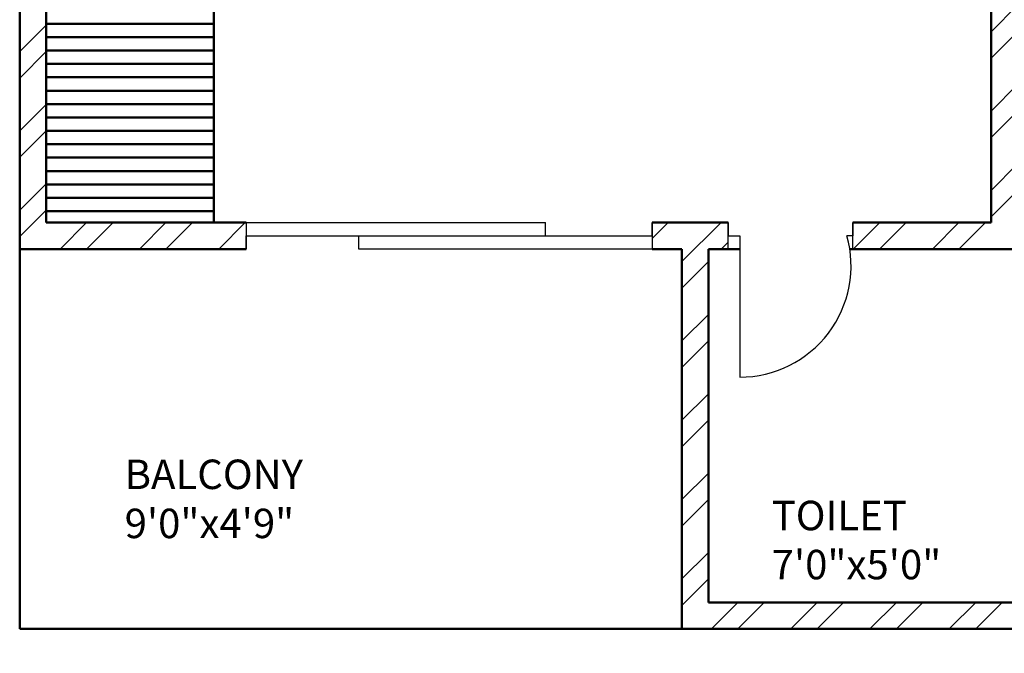
# Model space of a CAD drawing. Units: inches. Extents: x 963 to 2075, y 289 to 2657.
# Tile 1 of 98: x 1091 to 1259, y 1474 to 1582. Entities that reach past the tile are written whole.
import ezdxf

# ---------------------------------------------------------------- set-up
doc = ezdxf.new("R2010")
doc.units = ezdxf.units.IN
for name, color, linetype, lineweight in [('A-AREA-IDEN', 7, 'Continuous', 18), ('A-DOOR', 4, 'Continuous', 25), ('A-GLAZ', 3, 'Continuous', 25), ('A-WALL', 7, 'Continuous', 50), ('A-WALL-PATT', 8, 'Continuous', 13)]:
    doc.layers.add(name, color=color, linetype=linetype, lineweight=lineweight)
doc.styles.get("Standard").update_dxf_attribs({"font": 'arial.ttf'})

msp = doc.modelspace()

# ---------------------------------------------------------------- hatches: boundary and pattern name
at = {"layer": 'A-WALL-PATT'}
h = msp.add_hatch(dxfattribs=at)
h.set_pattern_fill('ANSI32', color=256)
h.paths.add_polyline_path([(1296.92, 2558.32), (1203.92, 2558.32), (1203.92, 2493.82), (1191.53, 2493.82), (1191.53, 2489.32), (1211.06, 2489.32), (1211.06, 2492.02), (1211.06, 2493.82), (1208.42, 2493.82), (1208.42, 2553.82), (1292.42, 2553.82), (1292.42, 2538.86), (1296.92, 2538.86)])
h.paths.add_polyline_path([(1442.42, 2558.32), (1349.42, 2558.32), (1349.42, 2538.94), (1353.92, 2538.94), (1353.92, 2553.82), (1437.92, 2553.82), (1437.92, 2493.82), (1434.54, 2493.82), (1434.54, 2489.32), (1448.31, 2489.32), (1448.31, 2491.57), (1448.31, 2493.82), (1442.42, 2493.82)])
h.paths.add_polyline_path([(1415.55, 2491.57), (1415.55, 2493.82), (1340.94, 2493.82), (1340.94, 2489.32), (1371.92, 2489.32), (1371.92, 2378.32), (1367.6, 2378.32), (1367.6, 2373.82), (1371.92, 2373.82), (1371.92, 2355.19), (1376.42, 2355.19), (1376.42, 2489.32), (1415.55, 2489.32)])
h.paths.add_polyline_path([(1304.94, 2491.57), (1304.94, 2493.82), (1296.92, 2493.82), (1296.92, 2514.86), (1292.42, 2514.86), (1292.42, 2493.82), (1232.81, 2493.82), (1232.81, 2489.32), (1256.42, 2489.32), (1256.42, 2327.32), (1253.71, 2327.32), (1253.71, 2322.82), (1328.42, 2322.82), (1328.42, 2331.15), (1323.92, 2331.15), (1323.92, 2327.32), (1260.92, 2327.32), (1260.92, 2373.82), (1323.92, 2373.82), (1323.92, 2357.81), (1328.42, 2357.81), (1328.42, 2373.82), (1346.01, 2373.82), (1346.01, 2376.07), (1346.01, 2378.32), (1260.92, 2378.32), (1260.92, 2489.32), (1304.94, 2489.32)])
h.paths.add_polyline_path([(1226.65, 2327.32), (1124.42, 2327.32), (1124.42, 2347.45), (1119.92, 2347.45), (1119.92, 2322.82), (1163.42, 2322.82), (1163.42, 2305.43), (1165.67, 2305.43), (1167.92, 2305.43), (1167.92, 2322.82), (1226.65, 2322.82), (1226.65, 2325.07)])
h.paths.add_polyline_path([(1095.92, 2489.32), (1124.42, 2489.32), (1131.53, 2489.32), (1131.53, 2491.57), (1131.53, 2493.82), (1119.92, 2493.82), (1091.42, 2493.82), (1091.42, 2417.32), (1095.92, 2417.32), (1119.92, 2417.32), (1119.92, 2407.45), (1124.42, 2407.45), (1124.42, 2421.82), (1095.92, 2421.82)])
h.paths.add_polyline_path([(1512.92, 2558.32), (1508.42, 2558.32), (1508.42, 2493.82), (1503.4, 2493.82), (1503.4, 2489.32), (1508.42, 2489.32), (1508.42, 2327.32), (1376.42, 2327.32), (1376.42, 2330.27), (1371.92, 2330.27), (1371.92, 2298.74), (1376.42, 2298.74), (1376.42, 2322.82), (1508.42, 2322.82), (1508.42, 2165.32), (1504.26, 2165.32), (1504.26, 2160.82), (1508.42, 2160.82), (1508.42, 2108.32), (1512.92, 2108.32), (1512.92, 2160.82), (1516.18, 2160.82), (1516.18, 2163.07), (1516.18, 2165.32), (1512.92, 2165.32), (1512.92, 2322.82), (1644.92, 2322.82), (1644.92, 2298.74), (1649.42, 2298.74), (1649.42, 2322.82), (1649.42, 2330.94), (1647.17, 2330.94), (1644.92, 2330.94), (1644.92, 2327.32), (1512.92, 2327.32), (1512.92, 2489.32), (1516.76, 2489.32), (1516.76, 2491.57), (1516.76, 2493.82), (1512.92, 2493.82)])
h.paths.add_polyline_path([(1671.92, 2558.32), (1578.92, 2558.32), (1578.92, 2493.82), (1573.53, 2493.82), (1573.53, 2489.32), (1586.54, 2489.32), (1586.54, 2491.57), (1586.54, 2493.82), (1583.42, 2493.82), (1583.42, 2553.82), (1667.42, 2553.82), (1667.42, 2541.11), (1671.92, 2541.11)])
h.paths.add_polyline_path([(1681.26, 2493.82), (1671.92, 2493.82), (1671.92, 2517.11), (1667.42, 2517.11), (1667.42, 2493.82), (1610.22, 2493.82), (1610.22, 2489.32), (1644.92, 2489.32), (1644.92, 2357.87), (1649.42, 2357.87), (1649.42, 2373.82), (1652.2, 2373.82), (1652.2, 2375.83), (1652.2, 2378.32), (1649.42, 2378.32), (1649.42, 2489.32), (1681.26, 2489.32), (1681.26, 2491.57)])
h.paths.add_polyline_path([(1821.92, 2558.32), (1728.92, 2558.32), (1728.92, 2541), (1733.42, 2541), (1733.42, 2553.82), (1817.42, 2553.82), (1817.42, 2493.82), (1813.51, 2493.82), (1813.51, 2489.32), (1830.08, 2489.32), (1830.08, 2491.57), (1830.08, 2493.82), (1821.92, 2493.82)])
h.paths.add_polyline_path([(1794.24, 2493.82), (1717.26, 2493.82), (1717.26, 2489.32), (1760.42, 2489.32), (1760.42, 2378.32), (1674.4, 2378.32), (1674.4, 2373.82), (1692.92, 2373.82), (1692.92, 2356.95), (1697.42, 2356.95), (1697.42, 2373.82), (1760.42, 2373.82), (1760.42, 2327.32), (1697.42, 2327.32), (1697.42, 2333.34), (1692.92, 2333.34), (1692.92, 2322.82), (1768.04, 2322.82), (1768.04, 2325.07), (1768.04, 2327.32), (1764.92, 2327.32), (1764.92, 2489.32), (1794.24, 2489.32)])
h.paths.add_polyline_path([(1733.42, 2517), (1728.92, 2517), (1728.92, 2493.82), (1733.42, 2493.82)], flags=17)
h.paths.add_polyline_path([(1929.92, 2493.82), (1890.08, 2493.82), (1890.08, 2489.32), (1896.92, 2489.32), (1925.42, 2489.32), (1925.42, 2421.82), (1896.92, 2421.82), (1896.92, 2408.32), (1901.42, 2408.32), (1901.42, 2417.32), (1925.42, 2417.32), (1929.92, 2417.32)])
h.paths.add_polyline_path([(1901.42, 2348.32), (1896.92, 2348.32), (1896.92, 2327.32), (1800.42, 2327.32), (1800.42, 2322.82), (1853.42, 2322.82), (1853.42, 2309.45), (1857.92, 2309.45), (1857.92, 2322.82), (1901.42, 2322.82)])
h.paths.add_polyline_path([(1857.92, 2249.45), (1853.42, 2249.45), (1853.42, 2214.82), (1686.31, 2214.82), (1686.31, 2210.32), (1853.42, 2210.32), (1853.42, 2202.13), (1857.92, 2202.13), (1857.92, 2210.32)])
h.paths.add_polyline_path([(1857.92, 2142.13), (1853.42, 2142.13), (1853.42, 2115.42), (1841.42, 2115.42), (1841.42, 2088.53), (1841.42, 2046.95), (1845.92, 2046.95), (1845.92, 2110.92), (1905.92, 2110.92), (1905.92, 2092.52), (1910.42, 2092.52), (1910.42, 2115.42), (1857.92, 2115.42)])
h.paths.add_polyline_path([(1532.44, 1482.34), (1573.46, 1482.34), (1573.46, 1501), (1532.44, 1501)], flags=9)
h.paths.add_polyline_path([(1438.66, 1486.3), (1479.68, 1486.3), (1479.68, 1504.96), (1438.66, 1504.96)], flags=9)
h.paths.add_polyline_path([(1411.22, 1365.31), (1659.14, 1365.31), (1659.14, 1402.4), (1411.22, 1402.4)], flags=9)
h.paths.add_polyline_path([(1185.67, 2296.3), (1248.16, 2296.3), (1248.16, 2314.95), (1185.67, 2314.95)], flags=9)
h.paths.add_polyline_path([(1177.31, 2187.35), (1216.15, 2187.35), (1216.15, 2206.01), (1177.31, 2206.01)], flags=9)
h.paths.add_polyline_path([(1295.1, 1602.08), (1328.26, 1602.08), (1328.26, 1620.74), (1295.1, 1620.74)], flags=9)
h.paths.add_polyline_path([(1525.13, 2005.99), (1558.39, 2005.99), (1558.39, 2024.65), (1525.13, 2024.65)], flags=9)
h.paths.add_polyline_path([(1459.61, 1977.13), (1472.19, 1977.13), (1472.19, 1987.43), (1459.61, 1987.43)], flags=9)
h.paths.add_polyline_path([(1467.81, 2053.68), (1480.02, 2053.68), (1480.02, 2063.98), (1467.81, 2063.98)], flags=9)
h.paths.add_polyline_path([(1555.18, 2119.02), (1584.56, 2119.02), (1584.56, 2137.68), (1555.18, 2137.68)], flags=25)
h.paths.add_polyline_path([(1405.39, 2115.29), (1444.48, 2115.29), (1444.48, 2133.95), (1405.39, 2133.95)], flags=25)
h.paths.add_polyline_path([(1698.48, 2004.26), (1727.69, 2004.26), (1727.69, 2022.92), (1698.48, 2022.92)], flags=9)
h.paths.add_polyline_path([(1612.16, 1972.86), (1629.02, 1972.86), (1629.02, 1983.16), (1612.16, 1983.16)], flags=9)
h.paths.add_polyline_path([(1608.29, 2060.04), (1625.15, 2060.04), (1625.15, 2070.34), (1608.29, 2070.34)], flags=9)
h.paths.add_polyline_path([(1527.95, 1684.4), (1566.79, 1684.4), (1566.79, 1703.06), (1527.95, 1703.06)], flags=9)
h.paths.add_polyline_path([(1422.79, 1683.59), (1461.63, 1683.59), (1461.63, 1702.25), (1422.79, 1702.25)], flags=9)
h.paths.add_polyline_path([(1531.26, 1732.46), (1574.01, 1732.46), (1574.01, 1751.12), (1531.26, 1751.12)], flags=9)
h.paths.add_polyline_path([(1402.87, 1732.85), (1439.8, 1732.85), (1439.8, 1751.5), (1402.87, 1751.5)], flags=9)
h.paths.add_polyline_path([(1243.12, 1923.13), (1281.96, 1923.13), (1281.96, 1941.79), (1243.12, 1941.79)], flags=9)
h.paths.add_polyline_path([(1181.75, 1792.27), (1244.24, 1792.27), (1244.24, 1810.93), (1181.75, 1810.93)], flags=9)
h.paths.add_polyline_path([(1265.82, 1670.3), (1316.07, 1670.3), (1316.07, 1688.96), (1265.82, 1688.96)], flags=9)
h.paths.add_polyline_path([(1140.26, 1676.05), (1179.1, 1676.05), (1179.1, 1694.71), (1140.26, 1694.71)], flags=9)
h.paths.add_polyline_path([(1107.49, 1490.89), (1143.37, 1490.89), (1143.37, 1509.55), (1107.49, 1509.55)], flags=9)
h.paths.add_polyline_path([(1217.58, 1483.9), (1246.74, 1483.9), (1246.74, 1502.56), (1217.58, 1502.56)], flags=9)
h.paths.add_polyline_path([(1389.21, 1486.92), (1418.37, 1486.92), (1418.37, 1505.58), (1389.21, 1505.58)], flags=9)
h.paths.add_polyline_path([(1672.21, 1602.08), (1705.37, 1602.08), (1705.37, 1620.74), (1672.21, 1620.74)], flags=9)
h.paths.add_polyline_path([(1752.08, 1522.64), (1781.24, 1522.64), (1781.24, 1541.3), (1752.08, 1541.3)], flags=9)
h.paths.add_polyline_path([(1848.27, 1491.26), (1884.16, 1491.26), (1884.16, 1509.92), (1848.27, 1509.92)], flags=9)
h.paths.add_polyline_path([(1822.47, 1685.62), (1861.31, 1685.62), (1861.31, 1704.28), (1822.47, 1704.28)], flags=9)
h.paths.add_polyline_path([(1713.19, 1672.23), (1763.44, 1672.23), (1763.44, 1690.89), (1713.19, 1690.89)], flags=9)
h.paths.add_polyline_path([(1736.62, 1790.58), (1799.11, 1790.58), (1799.11, 1809.24), (1736.62, 1809.24)], flags=9)
h.paths.add_polyline_path([(1691.49, 1916.36), (1730.33, 1916.36), (1730.33, 1935.01), (1691.49, 1935.01)], flags=9)
h.paths.add_polyline_path([(1764.87, 1973.92), (1794.31, 1973.92), (1794.31, 1992.58), (1764.87, 1992.58)], flags=9)
h.paths.add_polyline_path([(1767.85, 2034.02), (1797.29, 2034.02), (1797.29, 2052.67), (1767.85, 2052.67)], flags=9)
h.paths.add_polyline_path([(1851.59, 2060.33), (1880.75, 2060.33), (1880.75, 2078.99), (1851.59, 2078.99)], flags=25)
h.paths.add_polyline_path([(1688.49, 2086.87), (1727.33, 2086.87), (1727.33, 2105.53), (1688.49, 2105.53)], flags=9)
h.paths.add_polyline_path([(1537.74, 2293.58), (1580.49, 2293.58), (1580.49, 2312.24), (1537.74, 2312.24)], flags=25)
h.paths.add_polyline_path([(1425.59, 2296.11), (1468.34, 2296.11), (1468.34, 2314.77), (1425.59, 2314.77)], flags=25)
h.paths.add_polyline_path([(1278.52, 2004.18), (1307.72, 2004.18), (1307.72, 2022.84), (1278.52, 2022.84)], flags=9)
h.paths.add_polyline_path([(1193.28, 1973.63), (1222.72, 1973.63), (1222.72, 1992.29), (1193.28, 1992.29)], flags=9)
h.paths.add_polyline_path([(1192.41, 2040.58), (1221.84, 2040.58), (1221.84, 2059.23), (1192.41, 2059.23)], flags=9)
h.paths.add_polyline_path([(1130.6, 1951.39), (1159.76, 1951.39), (1159.76, 1970.05), (1130.6, 1970.05)], flags=9)
h.paths.add_polyline_path([(1132.83, 2052.49), (1161.98, 2052.49), (1161.98, 2071.15), (1132.83, 2071.15)], flags=9)
h.paths.add_polyline_path([(1265.13, 2334.62), (1315.38, 2334.62), (1315.38, 2353.28), (1265.13, 2353.28)], flags=25)
h.paths.add_polyline_path([(1136.74, 2330.79), (1175.58, 2330.79), (1175.58, 2349.44), (1136.74, 2349.44)], flags=9)
h.paths.add_polyline_path([(1287.42, 2417.2), (1320.58, 2417.2), (1320.58, 2435.86), (1287.42, 2435.86)], flags=25)
h.paths.add_polyline_path([(1430.99, 2329.16), (1469.83, 2329.16), (1469.83, 2347.82), (1430.99, 2347.82)], flags=25)
h.paths.add_polyline_path([(1525.42, 2329.21), (1564.26, 2329.21), (1564.26, 2347.87), (1525.42, 2347.87)], flags=25)
h.paths.add_polyline_path([(1684.52, 2382.8), (1717.68, 2382.8), (1717.68, 2401.46), (1684.52, 2401.46)], flags=25)
h.paths.add_polyline_path([(1704.81, 2340.29), (1755.05, 2340.29), (1755.05, 2358.95), (1704.81, 2358.95)], flags=25)
h.paths.add_polyline_path([(1694.11, 2287.76), (1756.6, 2287.76), (1756.6, 2306.41), (1694.11, 2306.41)], flags=9)
h.paths.add_polyline_path([(1815.78, 2329.86), (1854.62, 2329.86), (1854.62, 2348.52), (1815.78, 2348.52)], flags=9)
h.paths.add_polyline_path([(1842.87, 2514.26), (1878.76, 2514.26), (1878.76, 2532.91), (1842.87, 2532.91)], flags=9)
h.paths.add_polyline_path([(1769.51, 2531.45), (1798.67, 2531.45), (1798.67, 2550.1), (1769.51, 2550.1)], flags=25)
h.paths.add_polyline_path([(1594.77, 2518.47), (1623.93, 2518.47), (1623.93, 2537.13), (1594.77, 2537.13)], flags=25)
h.paths.add_polyline_path([(1520.72, 2516.18), (1556.61, 2516.18), (1556.61, 2534.84), (1520.72, 2534.84)], flags=25)
h.paths.add_polyline_path([(1464.46, 2516.69), (1500.34, 2516.69), (1500.34, 2535.35), (1464.46, 2535.35)], flags=25)
h.paths.add_polyline_path([(1365.7, 2528.97), (1394.85, 2528.97), (1394.85, 2547.63), (1365.7, 2547.63)], flags=25)
h.paths.add_polyline_path([(1222.84, 2516.23), (1252, 2516.23), (1252, 2534.89), (1222.84, 2534.89)], flags=25)
h.paths.add_polyline_path([(1104.55, 2509.6), (1140.43, 2509.6), (1140.43, 2528.26), (1104.55, 2528.26)], flags=9)
h = msp.add_hatch(dxfattribs=at)
h.set_pattern_fill('ANSI32', color=256)
h.paths.add_polyline_path([(1335.97, 2212.57), (1335.97, 2214.82), (1167.92, 2214.82), (1167.92, 2245.43), (1163.42, 2245.43), (1163.42, 2210.32), (1163.42, 2194.81), (1167.92, 2194.81), (1167.92, 2210.32), (1335.97, 2210.32)])
h.paths.add_polyline_path([(1532.44, 1482.34), (1573.46, 1482.34), (1573.46, 1501), (1532.44, 1501)], flags=9)
h.paths.add_polyline_path([(1438.66, 1486.3), (1479.68, 1486.3), (1479.68, 1504.96), (1438.66, 1504.96)], flags=9)
h.paths.add_polyline_path([(1411.22, 1365.31), (1659.14, 1365.31), (1659.14, 1402.4), (1411.22, 1402.4)], flags=9)
h.paths.add_polyline_path([(1185.67, 2296.3), (1248.16, 2296.3), (1248.16, 2314.95), (1185.67, 2314.95)], flags=9)
h.paths.add_polyline_path([(1177.31, 2187.35), (1216.15, 2187.35), (1216.15, 2206.01), (1177.31, 2206.01)], flags=9)
h.paths.add_polyline_path([(1295.1, 1602.08), (1328.26, 1602.08), (1328.26, 1620.74), (1295.1, 1620.74)], flags=9)
h.paths.add_polyline_path([(1525.13, 2005.99), (1558.39, 2005.99), (1558.39, 2024.65), (1525.13, 2024.65)], flags=9)
h.paths.add_polyline_path([(1459.61, 1977.13), (1472.19, 1977.13), (1472.19, 1987.43), (1459.61, 1987.43)], flags=9)
h.paths.add_polyline_path([(1467.81, 2053.68), (1480.02, 2053.68), (1480.02, 2063.98), (1467.81, 2063.98)], flags=9)
h.paths.add_polyline_path([(1555.18, 2119.02), (1584.56, 2119.02), (1584.56, 2137.68), (1555.18, 2137.68)], flags=9)
h.paths.add_polyline_path([(1405.39, 2115.29), (1444.48, 2115.29), (1444.48, 2133.95), (1405.39, 2133.95)], flags=9)
h.paths.add_polyline_path([(1698.48, 2004.26), (1727.69, 2004.26), (1727.69, 2022.92), (1698.48, 2022.92)], flags=9)
h.paths.add_polyline_path([(1612.16, 1972.86), (1629.02, 1972.86), (1629.02, 1983.16), (1612.16, 1983.16)], flags=9)
h.paths.add_polyline_path([(1608.29, 2060.04), (1625.15, 2060.04), (1625.15, 2070.34), (1608.29, 2070.34)], flags=9)
h.paths.add_polyline_path([(1527.95, 1684.4), (1566.79, 1684.4), (1566.79, 1703.06), (1527.95, 1703.06)], flags=9)
h.paths.add_polyline_path([(1422.79, 1683.59), (1461.63, 1683.59), (1461.63, 1702.25), (1422.79, 1702.25)], flags=9)
h.paths.add_polyline_path([(1531.26, 1732.46), (1574.01, 1732.46), (1574.01, 1751.12), (1531.26, 1751.12)], flags=9)
h.paths.add_polyline_path([(1402.87, 1732.85), (1439.8, 1732.85), (1439.8, 1751.5), (1402.87, 1751.5)], flags=9)
h.paths.add_polyline_path([(1243.12, 1923.13), (1281.96, 1923.13), (1281.96, 1941.79), (1243.12, 1941.79)], flags=9)
h.paths.add_polyline_path([(1181.75, 1792.27), (1244.24, 1792.27), (1244.24, 1810.93), (1181.75, 1810.93)], flags=9)
h.paths.add_polyline_path([(1265.82, 1670.3), (1316.07, 1670.3), (1316.07, 1688.96), (1265.82, 1688.96)], flags=9)
h.paths.add_polyline_path([(1140.26, 1676.05), (1179.1, 1676.05), (1179.1, 1694.71), (1140.26, 1694.71)], flags=9)
h.paths.add_polyline_path([(1107.49, 1490.89), (1143.37, 1490.89), (1143.37, 1509.55), (1107.49, 1509.55)], flags=9)
h.paths.add_polyline_path([(1217.58, 1483.9), (1246.74, 1483.9), (1246.74, 1502.56), (1217.58, 1502.56)], flags=9)
h.paths.add_polyline_path([(1389.21, 1486.92), (1418.37, 1486.92), (1418.37, 1505.58), (1389.21, 1505.58)], flags=9)
h.paths.add_polyline_path([(1672.21, 1602.08), (1705.37, 1602.08), (1705.37, 1620.74), (1672.21, 1620.74)], flags=9)
h.paths.add_polyline_path([(1752.08, 1522.64), (1781.24, 1522.64), (1781.24, 1541.3), (1752.08, 1541.3)], flags=9)
h.paths.add_polyline_path([(1848.27, 1491.26), (1884.16, 1491.26), (1884.16, 1509.92), (1848.27, 1509.92)], flags=9)
h.paths.add_polyline_path([(1822.47, 1685.62), (1861.31, 1685.62), (1861.31, 1704.28), (1822.47, 1704.28)], flags=9)
h.paths.add_polyline_path([(1713.19, 1672.23), (1763.44, 1672.23), (1763.44, 1690.89), (1713.19, 1690.89)], flags=9)
h.paths.add_polyline_path([(1736.62, 1790.58), (1799.11, 1790.58), (1799.11, 1809.24), (1736.62, 1809.24)], flags=9)
h.paths.add_polyline_path([(1691.49, 1916.36), (1730.33, 1916.36), (1730.33, 1935.01), (1691.49, 1935.01)], flags=9)
h.paths.add_polyline_path([(1764.87, 1973.92), (1794.31, 1973.92), (1794.31, 1992.58), (1764.87, 1992.58)], flags=9)
h.paths.add_polyline_path([(1767.85, 2034.02), (1797.29, 2034.02), (1797.29, 2052.67), (1767.85, 2052.67)], flags=9)
h.paths.add_polyline_path([(1851.59, 2060.33), (1880.75, 2060.33), (1880.75, 2078.99), (1851.59, 2078.99)], flags=9)
h.paths.add_polyline_path([(1688.49, 2086.87), (1727.33, 2086.87), (1727.33, 2105.53), (1688.49, 2105.53)], flags=9)
h.paths.add_polyline_path([(1537.74, 2293.58), (1580.49, 2293.58), (1580.49, 2312.24), (1537.74, 2312.24)], flags=9)
h.paths.add_polyline_path([(1425.59, 2296.11), (1468.34, 2296.11), (1468.34, 2314.77), (1425.59, 2314.77)], flags=9)
h.paths.add_polyline_path([(1278.52, 2004.18), (1307.72, 2004.18), (1307.72, 2022.84), (1278.52, 2022.84)], flags=9)
h.paths.add_polyline_path([(1193.28, 1973.63), (1222.72, 1973.63), (1222.72, 1992.29), (1193.28, 1992.29)], flags=9)
h.paths.add_polyline_path([(1192.41, 2040.58), (1221.84, 2040.58), (1221.84, 2059.23), (1192.41, 2059.23)], flags=9)
h.paths.add_polyline_path([(1130.6, 1951.39), (1159.76, 1951.39), (1159.76, 1970.05), (1130.6, 1970.05)], flags=9)
h.paths.add_polyline_path([(1132.83, 2052.49), (1161.98, 2052.49), (1161.98, 2071.15), (1132.83, 2071.15)], flags=9)
h.paths.add_polyline_path([(1265.13, 2334.62), (1315.38, 2334.62), (1315.38, 2353.28), (1265.13, 2353.28)], flags=9)
h.paths.add_polyline_path([(1136.74, 2330.79), (1175.58, 2330.79), (1175.58, 2349.44), (1136.74, 2349.44)], flags=9)
h.paths.add_polyline_path([(1287.42, 2417.2), (1320.58, 2417.2), (1320.58, 2435.86), (1287.42, 2435.86)], flags=9)
h.paths.add_polyline_path([(1430.99, 2329.16), (1469.83, 2329.16), (1469.83, 2347.82), (1430.99, 2347.82)], flags=9)
h.paths.add_polyline_path([(1525.42, 2329.21), (1564.26, 2329.21), (1564.26, 2347.87), (1525.42, 2347.87)], flags=9)
h.paths.add_polyline_path([(1684.52, 2382.8), (1717.68, 2382.8), (1717.68, 2401.46), (1684.52, 2401.46)], flags=9)
h.paths.add_polyline_path([(1704.81, 2340.29), (1755.05, 2340.29), (1755.05, 2358.95), (1704.81, 2358.95)], flags=9)
h.paths.add_polyline_path([(1694.11, 2287.76), (1756.6, 2287.76), (1756.6, 2306.41), (1694.11, 2306.41)], flags=9)
h.paths.add_polyline_path([(1815.78, 2329.86), (1854.62, 2329.86), (1854.62, 2348.52), (1815.78, 2348.52)], flags=9)
h.paths.add_polyline_path([(1842.87, 2514.26), (1878.76, 2514.26), (1878.76, 2532.91), (1842.87, 2532.91)], flags=9)
h.paths.add_polyline_path([(1769.51, 2531.45), (1798.67, 2531.45), (1798.67, 2550.1), (1769.51, 2550.1)], flags=9)
h.paths.add_polyline_path([(1594.77, 2518.47), (1623.93, 2518.47), (1623.93, 2537.13), (1594.77, 2537.13)], flags=9)
h.paths.add_polyline_path([(1520.72, 2516.18), (1556.61, 2516.18), (1556.61, 2534.84), (1520.72, 2534.84)], flags=9)
h.paths.add_polyline_path([(1464.46, 2516.69), (1500.34, 2516.69), (1500.34, 2535.35), (1464.46, 2535.35)], flags=9)
h.paths.add_polyline_path([(1365.7, 2528.97), (1394.85, 2528.97), (1394.85, 2547.63), (1365.7, 2547.63)], flags=9)
h.paths.add_polyline_path([(1222.84, 2516.23), (1252, 2516.23), (1252, 2534.89), (1222.84, 2534.89)], flags=9)
h.paths.add_polyline_path([(1104.55, 2509.6), (1140.43, 2509.6), (1140.43, 2528.26), (1104.55, 2528.26)], flags=9)
h = msp.add_hatch(dxfattribs=at)
h.set_pattern_fill('ANSI32', color=256)
h.paths.add_polyline_path([(1473.61, 2163.07), (1473.61, 2165.32), (1376.42, 2165.32), (1376.42, 2227.98), (1371.92, 2227.98), (1371.92, 2214.82), (1368.41, 2214.82), (1368.41, 2210.32), (1371.92, 2210.32), (1371.92, 2160.82), (1395.92, 2160.82), (1395.92, 2090.32), (1217.34, 2090.32), (1217.34, 2085.82), (1395.92, 2085.82), (1458.92, 2085.82), (1458.92, 2108.32), (1454.42, 2108.32), (1454.42, 2090.32), (1400.42, 2090.32), (1400.42, 2160.82), (1473.61, 2160.82)])
h.paths.add_polyline_path([(1649.42, 2210.32), (1653.23, 2210.32), (1653.23, 2214.82), (1649.42, 2214.82), (1649.42, 2227.98), (1644.92, 2227.98), (1644.92, 2165.32), (1550.1, 2165.32), (1550.1, 2160.82), (1620.92, 2160.82), (1620.92, 2112.82), (1555.45, 2112.82), (1555.45, 2108.32), (1584.33, 2108.32), (1584.33, 2084.92), (1588.83, 2084.92), (1588.83, 2108.32), (1625.42, 2108.32), (1667.95, 2108.32), (1667.95, 2022.67), (1588.83, 2022.67), (1588.83, 2047.41), (1584.33, 2047.41), (1584.33, 1996), (1588.83, 1996), (1588.83, 2018.32), (1667.95, 2018.17), (1667.95, 1928.32), (1625.42, 1928.32), (1625.42, 1923.82), (1672.45, 1923.82), (1672.45, 1928.32), (1672.45, 1946.66), (1785.45, 1946.66), (1785.45, 1951.16), (1743.03, 1951.16), (1743.03, 2017.92), (1841.42, 2017.92), (1841.42, 2014.77), (1845.92, 2014.77), (1845.92, 2017.92), (1905.92, 2017.92), (1905.92, 1987.51), (1910.42, 1987.51), (1910.42, 2022.42), (1910.42, 2068.52), (1905.92, 2068.52), (1905.92, 2022.42), (1845.92, 2022.42), (1845.92, 2025.85), (1843.67, 2025.85), (1841.42, 2025.85), (1841.42, 2022.42), (1743.03, 2022.42), (1743.03, 2084.03), (1768.45, 2084.03), (1785.45, 2084.03), (1785.45, 2088.53), (1672.45, 2088.53), (1672.45, 2112.82), (1667.95, 2112.82), (1625.42, 2112.82), (1625.42, 2160.82), (1649.42, 2160.82)])
h.paths.add_polyline_path([(1672.45, 2084.03), (1738.53, 2084.03), (1738.53, 1951.16), (1672.45, 1951.16)], flags=16)
h.paths.add_polyline_path([(1672.45, 2084.03), (1738.53, 2084.03), (1705.49, 2017.6)], flags=0)
h.paths.add_polyline_path([(1262.77, 2085.82), (1258.27, 2085.82), (1258.27, 2023.28), (1184.42, 2023.28), (1184.42, 2018.78), (1258.27, 2018.78), (1258.27, 1950.82), (1262.77, 1950.82)])
h.paths.add_polyline_path([(1312.27, 2085.82), (1307.77, 2085.82), (1307.77, 1950.82), (1312.27, 1950.82)])
h.paths.add_polyline_path([(1458.92, 1950.82), (1395.92, 1950.82), (1216.57, 1950.82), (1216.57, 1946.32), (1346.42, 1946.32), (1395.92, 1946.32), (1395.92, 1875.82), (1371.92, 1875.82), (1371.92, 1826.32), (1368.93, 1826.32), (1368.93, 1821.82), (1371.92, 1821.82), (1371.92, 1813.62), (1376.42, 1813.62), (1376.42, 1871.32), (1474.5, 1871.32), (1474.5, 1873.57), (1474.5, 1875.82), (1400.42, 1875.82), (1400.42, 1946.32), (1454.42, 1946.32), (1454.42, 1928.32), (1458.92, 1928.32)])
h.paths.add_polyline_path([(1184.42, 2120.78), (1167.92, 2120.78), (1167.92, 2134.81), (1165.67, 2134.81), (1163.42, 2134.81), (1163.42, 2120.78), (1119.92, 2120.78), (1119.92, 2098.1), (1124.42, 2098.1), (1124.42, 2116.28), (1167.92, 2116.28), (1179.92, 2116.28), (1179.92, 2045.92), (1184.42, 2045.92), (1184.42, 2090.32), (1184.42, 2116.28)])
h.paths.add_polyline_path([(1124.42, 2018.78), (1179.92, 2018.78), (1179.92, 2016.29), (1184.42, 2016.29), (1184.42, 2023.28), (1184.42, 2026.59), (1182.17, 2026.59), (1179.92, 2026.59), (1179.92, 2023.28), (1124.42, 2023.28), (1124.42, 2074.1), (1119.92, 2074.1), (1119.92, 2018.78), (1119.92, 1979.63), (1124.42, 1979.63)])
h.paths.add_polyline_path([(1184.42, 1925.78), (1184.42, 1946.32), (1184.42, 1996.07), (1182.17, 1996.07), (1179.92, 1996.07), (1179.92, 1925.78), (1124.42, 1925.78), (1124.42, 1955.63), (1119.92, 1955.5), (1119.92, 1921.28), (1158.92, 1921.28), (1158.92, 1909.98), (1163.42, 1909.98), (1163.42, 1921.28), (1184.42, 1921.28)])
h.paths.add_polyline_path([(1341.45, 1826.32), (1163.42, 1826.32), (1163.42, 1849.98), (1158.92, 1849.98), (1158.92, 1821.82), (1158.92, 1804.03), (1163.42, 1804.03), (1163.42, 1821.82), (1341.45, 1821.82)])
h.paths.add_polyline_path([(1222.98, 1713.82), (1163.42, 1713.82), (1163.42, 1744.03), (1161.17, 1744.03), (1158.92, 1744.03), (1158.92, 1713.82), (1119.92, 1713.82), (1119.92, 1694.65), (1124.42, 1694.65), (1124.42, 1709.32), (1158.92, 1709.32), (1222.98, 1709.32)])
h.paths.add_polyline_path([(1328.42, 1713.82), (1252.04, 1713.82), (1252.04, 1711.57), (1252.04, 1709.32), (1256.42, 1709.32), (1256.42, 1547.32), (1232.94, 1547.32), (1232.94, 1545.07), (1232.94, 1542.82), (1292.42, 1542.82), (1292.42, 1527.63), (1296.92, 1527.63), (1296.92, 1542.82), (1299.46, 1542.82), (1299.46, 1547.32), (1260.92, 1547.32), (1260.92, 1658.32), (1343.66, 1658.32), (1343.66, 1660.57), (1343.66, 1662.82), (1328.42, 1662.82), (1328.42, 1676.59), (1327.4, 1676.59), (1323.92, 1676.59), (1323.92, 1662.82), (1260.92, 1662.82), (1260.92, 1709.32), (1323.92, 1709.32), (1323.92, 1699.85), (1328.42, 1699.85)])
h.paths.add_polyline_path([(1649.42, 1875.82), (1625.42, 1875.82), (1625.42, 1928.32), (1620.92, 1928.32), (1588.83, 1928.32), (1588.83, 1950.59), (1584.33, 1950.59), (1584.33, 1928.32), (1555.45, 1928.32), (1555.45, 1923.82), (1620.92, 1923.82), (1620.92, 1875.82), (1548.95, 1875.82), (1548.95, 1873.57), (1548.95, 1871.32), (1644.92, 1871.32), (1644.92, 1813.62), (1649.42, 1813.62), (1649.42, 1821.82), (1652.04, 1821.82), (1652.04, 1824.07), (1652.04, 1826.32), (1649.42, 1826.32)])
h.paths.add_polyline_path([(1512.92, 1871.32), (1516.48, 1871.32), (1516.48, 1875.82), (1512.92, 1875.82), (1512.92, 1923.82), (1512.92, 1928.32), (1512.92, 1930.83), (1508.42, 1930.83), (1508.42, 1875.82), (1504.41, 1875.82), (1504.41, 1871.32), (1508.42, 1871.32), (1508.42, 1713.82), (1376.42, 1713.82), (1376.42, 1743.32), (1371.92, 1743.32), (1371.92, 1709.32), (1371.92, 1706.01), (1376.42, 1706.01), (1376.42, 1709.32), (1508.42, 1709.32), (1508.42, 1547.32), (1501.87, 1547.32), (1501.87, 1542.82), (1508.42, 1542.82), (1508.42, 1482.82), (1508.42, 1436.32), (1512.92, 1436.32), (1512.92, 1542.82), (1519.32, 1542.82), (1519.32, 1545.07), (1519.32, 1547.32), (1512.92, 1547.32), (1512.92, 1709.32), (1644.92, 1709.32), (1644.92, 1707.55), (1649.42, 1707.55), (1649.42, 1709.32), (1649.42, 1743.32), (1644.92, 1743.32), (1644.92, 1713.82), (1512.92, 1713.82)])
h.paths.add_polyline_path([(1129.88, 1545.07), (1129.88, 1547.32), (1124.42, 1547.32), (1095.92, 1547.32), (1095.92, 1614.82), (1124.42, 1614.82), (1124.42, 1619.32), (1095.92, 1619.32), (1091.42, 1619.32), (1091.42, 1542.82), (1095.92, 1542.82), (1119.92, 1542.82), (1129.88, 1542.82)])
h.paths.add_polyline_path([(1208.42, 1542.82), (1211.74, 1542.82), (1211.74, 1547.32), (1198.85, 1547.32), (1198.85, 1542.82), (1203.92, 1542.82), (1203.92, 1478.32), (1208.42, 1478.32), (1296.92, 1478.32), (1296.92, 1503.63), (1292.42, 1503.63), (1292.42, 1482.82), (1208.42, 1482.82)])
h.paths.add_polyline_path([(1430.42, 1542.82), (1435.7, 1542.82), (1435.7, 1545.07), (1435.7, 1547.32), (1422.66, 1547.32), (1422.66, 1545.07), (1422.66, 1542.82), (1425.92, 1542.82), (1425.92, 1482.86), (1341.92, 1482.86), (1341.92, 1502.73), (1337.42, 1502.73), (1337.42, 1478.36), (1425.92, 1478.36), (1425.92, 1440.82), (1425.92, 1436.32), (1430.42, 1436.32)])
h.paths.add_polyline_path([(1698.48, 2004.26), (1727.69, 2004.26), (1727.69, 2022.92), (1698.48, 2022.92)], flags=8)

# ---------------------------------------------------------------- linework, layer by layer
at = {"layer": 'A-DOOR'}
for p, q in [((1211.74, 1542.82), (1211.74, 1547.32)), ((1211.74, 1547.32), (1211.74, 1545.07)), ((1232.94, 1542.82), (1232.94, 1547.32)), ((1232.94, 1547.32), (1232.94, 1545.07)), ((1211.74, 1545.07), (1213.74, 1545.07)), ((1213.74, 1545.07), (1213.74, 1521.07)), ((1232.94, 1545.07), (1231.94, 1545.07))]:
    msp.add_line(p, q, dxfattribs=at)
msp.add_arc((1213.74, 1539.97), 18.9, 270, 15.6625, dxfattribs=at)
at = {"layer": 'A-GLAZ'}
for p, q in [((1129.88, 1547.32), (1129.88, 1542.82)), ((1129.88, 1547.32), (1180.76, 1547.32)), ((1180.76, 1545.07), (1180.76, 1547.32)), ((1198.85, 1545.07), (1198.85, 1547.32)), ((1198.85, 1547.32), (1198.85, 1542.82)), ((1129.88, 1542.82), (1129.88, 1545.07)), ((1129.88, 1545.07), (1198.85, 1545.07)), ((1149.01, 1542.82), (1149.01, 1545.07)), ((1198.85, 1542.82), (1149.01, 1542.82))]:
    msp.add_line(p, q, dxfattribs=at)
at = {"layer": 'A-WALL'}
for p, q in [((1256.42, 1709.32), (1256.42, 1547.32)), ((1124.42, 1634.65), (1124.42, 1547.32)), ((1124.42, 1634.65), (1124.42, 1547.32)), ((1091.42, 1619.32), (1091.42, 1542.82)), ((1095.92, 1547.32), (1095.92, 1614.82)), ((1124.42, 1581.07), (1095.92, 1581.07)), ((1124.42, 1578.8), (1095.92, 1578.8)), ((1124.42, 1576.53), (1095.92, 1576.53)), ((1124.42, 1574.25), (1095.92, 1574.25)), ((1124.42, 1571.98), (1095.92, 1571.98)), ((1124.42, 1569.71), (1095.92, 1569.71)), ((1124.42, 1567.43), (1095.92, 1567.43)), ((1124.42, 1565.16), (1095.92, 1565.16)), ((1124.42, 1562.88), (1095.92, 1562.88)), ((1124.42, 1560.61), (1095.92, 1560.61)), ((1124.42, 1558.34), (1095.92, 1558.34)), ((1124.42, 1556.06), (1095.92, 1556.06)), ((1124.42, 1553.79), (1095.92, 1553.79)), ((1124.42, 1551.52), (1095.92, 1551.52)), ((1124.42, 1549.24), (1095.92, 1549.24)), ((1124.42, 1547.32), (1095.92, 1547.32)), ((1124.42, 1547.32), (1129.88, 1547.32)), ((1198.85, 1547.32), (1211.74, 1547.32)), ((1232.94, 1547.32), (1256.42, 1547.32)), ((1091.42, 1542.82), (1095.92, 1542.82)), ((1091.42, 1542.82), (1091.42, 1478.32)), ((1119.92, 1542.82), (1095.92, 1542.82)), ((1129.88, 1542.82), (1119.92, 1542.82)), ((1203.92, 1542.82), (1198.85, 1542.82)), ((1203.92, 1542.82), (1203.92, 1478.32)), ((1208.42, 1542.82), (1208.42, 1482.82)), ((1213.74, 1542.82), (1208.42, 1542.82)), ((1292.42, 1542.82), (1232.42, 1542.82)), ((1208.42, 1482.82), (1292.42, 1482.82)), ((1091.42, 1478.32), (1208.42, 1478.32)), ((1296.92, 1478.32), (1208.42, 1478.32))]:
    msp.add_line(p, q, dxfattribs=at)

# ---------------------------------------------------------------- texts
at = {"layer": 'A-AREA-IDEN', "char_height": 5, "attachment_point": 1}
for s, width, insert in [('BALCONY\\P9\'0"x4\'9"', 195.5498, (1109.25, 1507.06)), ('TOILET\\P7\'0"x5\'0"', 127.6241, (1219.16, 1500.07))]:
    msp.add_mtext_dynamic_manual_height_columns(s, width=width, gutter_width=12.5, heights=[0], dxfattribs=dict(at, insert=insert))

doc.saveas('drawing.dxf')
